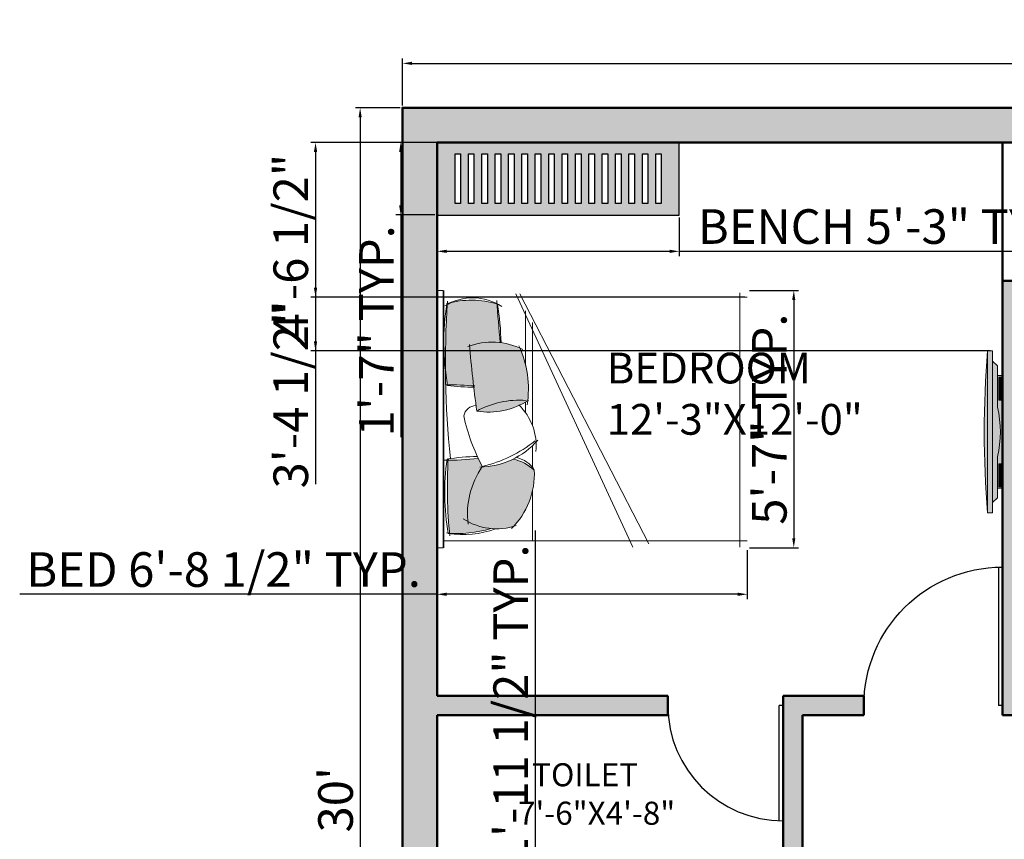
# Model space of a CAD drawing. Units: inches. Extents: x 3274 to 5176, y 1085 to 2172.
# Tile 6 of 16: x 3274 to 3530, y 1844 to 2057. Entities that reach past the tile are written whole.
import ezdxf

# ---------------------------------------------------------------- set-up
doc = ezdxf.new("R2010")
doc.units = ezdxf.units.IN
for name, color, linetype, lineweight in [('0.10', 252, 'Continuous', 9), ('A-ANNO-DIMS', 2, 'Continuous', 18), ('A-AREA-IDEN', 3, 'Continuous', 25), ('A-DOOR', 4, 'Continuous', 25), ('A-EQPM', 8, 'Continuous', 18), ('A-FLOR-PATT', 252, 'Continuous', 13), ('A-FURN', 8, 'Continuous', 18), ('A-WALL', 7, 'Continuous', 50), ('A-WALL-PATT', 8, 'Continuous', 13), ('moveis', 254, 'Continuous', 5), ('parede', 7, 'Continuous', 30)]:
    doc.layers.add(name, color=color, linetype=linetype, lineweight=lineweight)
doc.layers.add('MESA', color=7, linetype='Continuous')
doc.styles.get("Standard").update_dxf_attribs({"font": 'arial.ttf'})
doc.dimstyles.new('ISO-25', dxfattribs={"dimtxt": 9, "dimasz": 2.5, "dimexe": 1.25, "dimexo": 0.625, "dimtad": 1, "dimdec": 1, "dimlunit": 3, "dimtxsty": 'Standard', "dimcen": 2.5, "dimclrd": 4, "dimclre": 4, "dimclrt": 1, "dimadec": 0, "dimazin": 0, "dimtfac": 1, "dimtdec": 1, "dimtmove": 0, "dimatfit": 3, "dimfxl": 1, "dimarcsym": 0})

# ---------------------------------------------------------------- blocks, each defined once
blk = doc.blocks.new('1')
for p, q in [((0, 36), (0, 0)), ((1, 36), (1, 0)), ((0, 0), (1, 0))]:
    blk.add_line(p, q)
blk.add_arc((0, 0), 36, 0, 90)
blk = doc.blocks.new('2')
for p, q in [((0, 30), (0, 0)), ((1, 30), (1, 0)), ((0, 0), (1, 0))]:
    blk.add_line(p, q)
blk.add_arc((0, 0), 30, 0, 90)
blk = doc.blocks.new('*D67')
at = {"layer": 'A-ANNO-DIMS', "color": 0, "lineweight": -2, "transparency": 16777216}
for p, q in [((3373.3, 2035.11), (3373.3, 2047.29)), ((3375.8, 2046.04), (3730.8, 2046.04)), ((3733.3, 2035.11), (3733.3, 2047.29))]:
    blk.add_line(p, q, dxfattribs=at)
at = {"layer": 'A-ANNO-DIMS', "color": 0, "transparency": 16777216}
for points in [[(3375.8, 2046.46), (3375.8, 2045.63), (3373.3, 2046.04)], [(3730.8, 2046.46), (3730.8, 2045.63), (3733.3, 2046.04)]]:
    blk.add_solid(points, dxfattribs=at)
at = {"layer": 'Defpoints', "color": 0, "transparency": 16777216}
for p in [(3733.3, 2046.04), (3373.3, 2034.48), (3733.3, 2034.48)]:
    blk.add_point(p, dxfattribs=at)
at = {"layer": 'A-ANNO-DIMS', "color": 0, "transparency": 16777216, "insert": (3553.3, 2051.27), "char_height": 9, "attachment_point": 5}
blk.add_mtext("30'", dxfattribs=at)
blk = doc.blocks.new('*D68')
at = {"layer": 'A-ANNO-DIMS', "color": 0, "lineweight": -2, "transparency": 16777216}
for p, q in [((3372.68, 2034.48), (3361.05, 2034.48)), ((3362.3, 2031.98), (3362.3, 1676.98)), ((3372.68, 1674.48), (3361.05, 1674.48))]:
    blk.add_line(p, q, dxfattribs=at)
at = {"layer": 'A-ANNO-DIMS', "color": 0, "transparency": 16777216}
for points in [[(3361.88, 2031.98), (3362.71, 2031.98), (3362.3, 2034.48)], [(3361.88, 1676.98), (3362.71, 1676.98), (3362.3, 1674.48)]]:
    blk.add_solid(points, dxfattribs=at)
at = {"layer": 'Defpoints', "color": 0, "transparency": 16777216}
for p in [(3373.3, 2034.48), (3362.3, 1674.48), (3373.3, 1674.48)]:
    blk.add_point(p, dxfattribs=at)
at = {"layer": 'A-ANNO-DIMS', "color": 0, "transparency": 16777216, "insert": (3357.07, 1854.48), "char_height": 9, "attachment_point": 5, "rotation": 90}
blk.add_mtext("30'", dxfattribs=at)
blk = doc.blocks.new('camita')
at = {"layer": '0.10'}
for p, q in [((-0.85, -0.045), (0.85, -0.045)), ((-0.805, -0.045), (-0.805, -2.0485)), ((0.805, -0.045), (0.805, -2.0485)), ((-0.8271, -0.521), (0.8464, -1.2932)), ((-0.8271, -0.5476), (0.8236, -1.3992)), ((-0.7161, -0.585), (-0.3554, -0.585)), ((-0.1136, -0.585), (-0.0485, -0.585)), ((-0.638, -0.63), (0.0434, -0.63)), ((0.1749, -0.63), (0.3179, -0.63)), ((0.4739, -0.63), (0.805, -0.63)), ((-0.8354, -2), (0.8464, -2))]:
    blk.add_line(p, q, dxfattribs=at)
blk.add_lwpolyline([(-0.85, -0.0405), (0.85, -0.0405), (0.85, 0), (-0.85, 0)], close=True, dxfattribs=at)
for centre, radius, start, end in [((-0.4574, -0.2364), 0.3443, 147.50996, 213.83359), ((-0.1997, -0.2266), 0.5864, 163.92635, 197.14087), ((-0.3639, -5.8457), 5.7909, 83.80731, 94.12107), ((-0.5104, -1.7232), 1.6781, 80.12554, 98.66187), ((2.3534, -0.0532), 2.5803, 180.10628, 184.38541), ((-1.4396, -0.0609), 1.7117, 352.92911, 0.39592), ((0.4863, -1.6286), 1.5781, 80.16015, 98.05996), ((0.0294, -0.1377), 0.7262, 342.58415, 6.00484), ((-1.5443, -0.2452), 1.3333, 359.93941, 7.55329), ((1.5815, -0.2893), 1.3353, 170.38021, 178.99138), ((0.4524, -3.0675), 2.9996, 83.90257, 93.67595), ((0.1326, -0.1696), 0.6307, 339.92303, 8.74334), ((-0.007, -0.258), 0.0828, 100.01798, 179.73597), ((-0.2931, -1.4378), 1.2903, 61.97485, 77.84351), ((0.3203, -0.3944), 0.4043, 341.45245, 33.45121), ((-0.0543, -0.3633), 0.4542, 159.30257, 206.50263), ((-1.3301, -9.6748), 9.4985, 82.27078, 84.93989), ((0.6265, -0.7518), 0.5508, 82.96906, 124.67388), ((0.4585, -0.5454), 0.5842, 151.04555, 184.14969), ((-0.5341, -0.3393), 0.4875, 327.26442, 9.0473), ((-0.1986, -0.2742), 0.5159, 310.73945, 359.05759), ((-0.5673, -0.0868), 0.9057, 321.69527, 346.46261), ((-1.8672, -14.986), 14.6323, 84.65974, 85.75157), ((-0.4598, 1.4861), 1.9092, 260.95299, 268.65169), ((0.5707, -0.4317), 0.3145, 192.93877, 221.96363), ((0.3612, -0.133), 0.5096, 267.25889, 315.29965), ((-0.2002, 0.064), 0.6673, 244.78094, 279.06058), ((0.179, -0.272), 0.3828, 224.52836, 275.22287), ((0.4384, -0.4834), 0.1898, 193.68485, 236.70352)]:
    blk.add_arc(centre, radius, start, end, dxfattribs=at)
blk = doc.blocks.new('Banco Lintz')
at = {"layer": 'MESA', "ltscale": 0.05}
h = blk.add_hatch(color=256, dxfattribs=at)
h.dxf.hatch_style = 1
h.set_gradient(color1=(138, 84, 66), color2=(0, 0, 0), one_color=1, name='INVCYLINDER')
h.paths.add_polyline_path([(0.48, 0), (0, 0), (0, -1.6), (0.48, -1.6)])
h.paths.add_polyline_path([(0.4034, -0.5091), (0.0766, -0.5091), (0.0766, -0.4724), (0.4034, -0.4724)], flags=16)
h.paths.add_polyline_path([(0.4034, -0.5608), (0.4034, -0.5974), (0.0766, -0.5974), (0.0766, -0.5608)], flags=16)
h.paths.add_polyline_path([(0.4034, -0.4207), (0.0766, -0.4207), (0.0766, -0.384), (0.4034, -0.384)], flags=16)
h.paths.add_polyline_path([(0.4034, -0.6491), (0.4034, -0.6858), (0.0766, -0.6858), (0.0766, -0.6491)], flags=16)
h.paths.add_polyline_path([(0.4034, -0.3323), (0.0766, -0.3323), (0.0766, -0.2957), (0.4034, -0.2957)], flags=16)
h.paths.add_polyline_path([(0.4034, -0.7375), (0.4034, -0.7741), (0.0766, -0.7741), (0.0766, -0.7375)], flags=16)
h.paths.add_polyline_path([(0.4034, -0.244), (0.0766, -0.244), (0.0766, -0.2073), (0.4034, -0.2073)], flags=16)
h.paths.add_polyline_path([(0.4034, -0.8259), (0.4034, -0.8625), (0.0766, -0.8625), (0.0766, -0.8259)], flags=16)
h.paths.add_polyline_path([(0.4034, -0.1556), (0.0766, -0.1556), (0.0766, -0.119), (0.4034, -0.119)], flags=16)
h.paths.add_polyline_path([(0.4034, -0.9142), (0.4034, -0.9509), (0.0766, -0.9509), (0.0766, -0.9142)], flags=16)
h.paths.add_polyline_path([(0.4034, -1.0026), (0.4034, -1.0392), (0.0766, -1.0392), (0.0766, -1.0026)], flags=16)
h.paths.add_polyline_path([(0.4034, -1.0909), (0.4034, -1.1276), (0.0766, -1.1276), (0.0766, -1.0909)], flags=16)
h.paths.add_polyline_path([(0.4034, -1.1793), (0.4034, -1.216), (0.0766, -1.216), (0.0766, -1.1793)], flags=16)
h.paths.add_polyline_path([(0.4034, -1.2677), (0.4034, -1.3043), (0.0766, -1.3043), (0.0766, -1.2677)], flags=16)
h.paths.add_polyline_path([(0.4034, -1.356), (0.4034, -1.3927), (0.0766, -1.3927), (0.0766, -1.356)], flags=16)
h.paths.add_polyline_path([(0.4034, -1.4444), (0.4034, -1.481), (0.0766, -1.481), (0.0766, -1.4444)], flags=16)
for points in [[(0, -1.6), (0.48, -1.6), (0.48, 0), (0, 0)], [(0.0766, -0.119), (0.4034, -0.119), (0.4034, -0.1556), (0.0766, -0.1556)], [(0.0766, -0.2073), (0.4034, -0.2073), (0.4034, -0.244), (0.0766, -0.244)], [(0.0766, -0.2957), (0.4034, -0.2957), (0.4034, -0.3323), (0.0766, -0.3323)], [(0.0766, -0.384), (0.4034, -0.384), (0.4034, -0.4207), (0.0766, -0.4207)], [(0.0766, -0.4724), (0.4034, -0.4724), (0.4034, -0.5091), (0.0766, -0.5091)], [(0.0766, -0.5608), (0.4034, -0.5608), (0.4034, -0.5974), (0.0766, -0.5974)], [(0.0766, -0.6491), (0.4034, -0.6491), (0.4034, -0.6858), (0.0766, -0.6858)], [(0.0766, -0.7375), (0.4034, -0.7375), (0.4034, -0.7741), (0.0766, -0.7741)], [(0.0766, -0.8259), (0.4034, -0.8259), (0.4034, -0.8625), (0.0766, -0.8625)], [(0.0766, -0.9142), (0.4034, -0.9142), (0.4034, -0.9509), (0.0766, -0.9509)], [(0.0766, -1.0026), (0.4034, -1.0026), (0.4034, -1.0392), (0.0766, -1.0392)], [(0.0766, -1.0909), (0.4034, -1.0909), (0.4034, -1.1276), (0.0766, -1.1276)], [(0.0766, -1.1793), (0.4034, -1.1793), (0.4034, -1.216), (0.0766, -1.216)], [(0.0766, -1.2677), (0.4034, -1.2677), (0.4034, -1.3043), (0.0766, -1.3043)], [(0.0766, -1.356), (0.4034, -1.356), (0.4034, -1.3927), (0.0766, -1.3927)], [(0.0766, -1.4444), (0.4034, -1.4444), (0.4034, -1.481), (0.0766, -1.481)]]:
    blk.add_lwpolyline(points, close=True, dxfattribs=at)
blk = doc.blocks.new('PLASMA 2')
at = {"layer": 'moveis', "ltscale": 0.08}
h = blk.add_hatch(dxfattribs=at)
h.set_pattern_fill('_USER,_O', color=256, scale=0.008, double=1, pattern_type=0)
h.set_pattern_definition([(360, (-4.134502, -6.848382), (0, 0.008), []), (90, (-4.134502, -6.848382), (-0.008, 0), [])])
h.paths.add_polyline_path([(-0.2099, -0.0965), (-0.3623, -0.0965), (-0.3623, -0.1111), (-0.2099, -0.1111)])
h = blk.add_hatch(dxfattribs=at)
h.set_pattern_fill('_USER,_O', color=256, scale=0.008, double=1, pattern_type=0)
h.set_pattern_definition([(180, (4.134502, -6.848382), (0, 0.008), []), (90, (4.134502, -6.848382), (0.008, 0), [])])
h.paths.add_polyline_path([(0.2099, -0.0965), (0.3623, -0.0965), (0.3623, -0.1111), (0.2099, -0.1111)])
at = {"layer": 'parede', "ltscale": 0.08}
h = blk.add_hatch(color=256, dxfattribs=at)
h.dxf.hatch_style = 1
h.set_gradient(color1=(131, 136, 145), one_color=1, tint=1, name='CURVED')
h.paths.add_polyline_path([(-0.535, -0.0215), (0.535, -0.0215, 0.040195)])
h = blk.add_hatch(color=256, dxfattribs=at)
h.dxf.hatch_style = 1
h.set_gradient(color1=(131, 136, 145), color2=(0, 0, 0), one_color=1, name='CURVED')
h.paths.add_polyline_path([(0.535, -0.0215), (-0.535, -0.0215), (-0.535, -0.0553), (0.535, -0.0553)])
h = blk.add_hatch(color=256, dxfattribs=at)
h.dxf.hatch_style = 1
h.set_gradient(color1=(131, 136, 145), one_color=1, tint=1, name='CYLINDER')
h.paths.add_polyline_path([(0.4673, -0.0553), (-0.4673, -0.0553), (-0.4363, -0.0876), (-0.1636, -0.0876, 0.114423), (0.1636, -0.0876), (0.4363, -0.0876)])
h = blk.add_hatch(color=256, dxfattribs=at)
h.dxf.hatch_style = 1
h.set_gradient(color1=(131, 136, 145), color2=(0, 0, 0), one_color=1, name='CURVED')
h.paths.add_polyline_path([(0.3724, -0.0876), (0.1636, -0.0876, -0.114423), (-0.1636, -0.0876), (-0.3724, -0.0876), (-0.3724, -0.12), (0.3724, -0.12)])
h.paths.add_polyline_path([(-0.2099, -0.1111), (-0.3623, -0.1111), (-0.3623, -0.0965), (-0.2099, -0.0965)], flags=16)
h.paths.add_polyline_path([(0.2099, -0.1111), (0.2099, -0.0965), (0.3623, -0.0965), (0.3623, -0.1111)], flags=16)
at = {"layer": 'moveis', "ltscale": 0.08}
for p, q in [((-0.535, -0.0215), (-0.535, -0.0553)), ((-0.535, -0.0215), (0.535, -0.0215)), ((0.535, -0.0553), (-0.535, -0.0553)), ((-0.4673, -0.0553), (-0.4363, -0.0876)), ((0.4673, -0.0553), (0.4363, -0.0876)), ((0.535, -0.0553), (0.535, -0.0215)), ((-0.4363, -0.0876), (-0.1636, -0.0876)), ((-0.3724, -0.0876), (-0.3724, -0.12)), ((-0.3724, -0.12), (0.3724, -0.12)), ((0.1636, -0.0876), (0.4363, -0.0876)), ((0.3724, -0.0876), (0.3724, -0.12))]:
    blk.add_line(p, q, dxfattribs=at)
for points in [[(-0.3623, -0.0965), (-0.2099, -0.0965), (-0.2099, -0.1111), (-0.3623, -0.1111)], [(0.3623, -0.0965), (0.2099, -0.0965), (0.2099, -0.1111), (0.3623, -0.1111)]]:
    blk.add_lwpolyline(points, close=True, dxfattribs=at)
for centre, radius, start, end in [((0, -6.6658), 6.6658, 85.39647, 94.60353), ((0, 0.6178), 0.7242, 256.94486, 283.05514)]:
    blk.add_arc(centre, radius, start, end, dxfattribs=at)
blk = doc.blocks.new('*D132')
at = {"layer": 'A-ANNO-DIMS', "color": 4, "lineweight": -2, "transparency": 16777216}
for p, q in [((3382.3, 1919.39), (3382.3, 1906.67)), ((3462.96, 1919.39), (3462.96, 1906.67)), ((3382.3, 1907.92), (3273.77, 1907.92)), ((3460.46, 1907.92), (3384.8, 1907.92))]:
    blk.add_line(p, q, dxfattribs=at)
at = {"layer": 'A-ANNO-DIMS', "color": 4, "transparency": 16777216}
for points in [[(3384.8, 1908.33), (3384.8, 1907.5), (3382.3, 1907.92)], [(3460.46, 1908.33), (3460.46, 1907.5), (3462.96, 1907.92)]]:
    blk.add_solid(points, dxfattribs=at)
at = {"layer": 'Defpoints', "color": 0, "transparency": 16777216}
for p in [(3382.3, 1920.01), (3462.96, 1920.01), (3382.3, 1907.92)]:
    blk.add_point(p, dxfattribs=at)
at = {"layer": 'A-ANNO-DIMS', "color": 1, "transparency": 16777216, "insert": (3326.79, 1913.19), "char_height": 9, "attachment_point": 5}
blk.add_mtext('BED 6\'-8 1/2" TYP.', dxfattribs=at)
blk = doc.blocks.new('*D133')
at = {"layer": 'A-ANNO-DIMS', "color": 4, "lineweight": -2, "transparency": 16777216}
for p, q in [((3463.58, 1986.95), (3476.31, 1986.95)), ((3475.06, 1984.45), (3475.06, 1922.51)), ((3463.58, 1920.01), (3476.31, 1920.01))]:
    blk.add_line(p, q, dxfattribs=at)
at = {"layer": 'A-ANNO-DIMS', "color": 4, "transparency": 16777216}
for points in [[(3474.64, 1984.45), (3475.47, 1984.45), (3475.06, 1986.95)], [(3474.64, 1922.51), (3475.47, 1922.51), (3475.06, 1920.01)]]:
    blk.add_solid(points, dxfattribs=at)
at = {"layer": 'Defpoints', "color": 0, "transparency": 16777216}
for p in [(3462.96, 1986.95), (3462.96, 1920.01), (3475.06, 1920.01)]:
    blk.add_point(p, dxfattribs=at)
at = {"layer": 'A-ANNO-DIMS', "color": 1, "transparency": 16777216, "insert": (3469.86, 1953.48), "char_height": 9, "attachment_point": 5, "rotation": 90}
blk.add_mtext('5\'-7" TYP.', dxfattribs=at)
blk = doc.blocks.new('*D144')
at = {"layer": 'A-ANNO-DIMS', "color": 4, "lineweight": -2, "transparency": 16777216}
for p, q in [((3382.3, 2005.96), (3382.3, 1995.89)), ((3445.29, 2005.96), (3445.29, 1995.89)), ((3384.8, 1997.14), (3442.79, 1997.14)), ((3445.29, 1997.14), (3551.01, 1997.14))]:
    blk.add_line(p, q, dxfattribs=at)
at = {"layer": 'A-ANNO-DIMS', "color": 4, "transparency": 16777216}
for points in [[(3384.8, 1997.55), (3384.8, 1996.72), (3382.3, 1997.14)], [(3442.79, 1997.55), (3442.79, 1996.72), (3445.29, 1997.14)]]:
    blk.add_solid(points, dxfattribs=at)
at = {"layer": 'Defpoints', "color": 0, "transparency": 16777216}
for p in [(3382.3, 2006.59), (3445.29, 2006.59), (3445.29, 1997.14)]:
    blk.add_point(p, dxfattribs=at)
at = {"layer": 'A-ANNO-DIMS', "color": 1, "transparency": 16777216, "insert": (3499.4, 2002.42), "char_height": 9, "attachment_point": 5}
blk.add_mtext('BENCH 5\'-3" TYP.', dxfattribs=at)
blk = doc.blocks.new('*D145')
at = {"layer": 'A-ANNO-DIMS', "color": 4, "lineweight": -2, "transparency": 16777216}
for p, q in [((3381.68, 2025.48), (3371.6, 2025.48)), ((3372.85, 2022.98), (3372.85, 2009.09)), ((3381.68, 2006.59), (3371.6, 2006.59)), ((3372.85, 2006.59), (3372.85, 1948.82))]:
    blk.add_line(p, q, dxfattribs=at)
at = {"layer": 'A-ANNO-DIMS', "color": 4, "transparency": 16777216}
for points in [[(3372.44, 2022.98), (3373.27, 2022.98), (3372.85, 2025.48)], [(3372.44, 2009.09), (3373.27, 2009.09), (3372.85, 2006.59)]]:
    blk.add_solid(points, dxfattribs=at)
at = {"layer": 'Defpoints', "color": 0, "transparency": 16777216}
for p in [(3382.3, 2025.48), (3372.85, 2006.59), (3382.3, 2006.59)]:
    blk.add_point(p, dxfattribs=at)
at = {"layer": 'A-ANNO-DIMS', "color": 1, "transparency": 16777216, "insert": (3367.71, 1976.45), "char_height": 9, "attachment_point": 5, "rotation": 90}
blk.add_mtext('1\'-7" TYP.', dxfattribs=at)
blk = doc.blocks.new('*D146')
at = {"layer": 'A-ANNO-DIMS', "color": 4, "lineweight": -2, "transparency": 16777216}
for p, q in [((3407.89, 1746.82), (3407.89, 1924.51)), ((3404.98, 1746.82), (3409.14, 1746.82)), ((3407.89, 1725.73), (3407.89, 1744.32)), ((3404.98, 1723.23), (3409.14, 1723.23))]:
    blk.add_line(p, q, dxfattribs=at)
at = {"layer": 'A-ANNO-DIMS', "color": 4, "transparency": 16777216}
for points in [[(3407.48, 1744.32), (3408.31, 1744.32), (3407.89, 1746.82)], [(3407.48, 1725.73), (3408.31, 1725.73), (3407.89, 1723.23)]]:
    blk.add_solid(points, dxfattribs=at)
at = {"layer": 'Defpoints', "color": 0, "transparency": 16777216}
for p in [(3404.36, 1746.82), (3407.89, 1746.82), (3404.36, 1723.23)]:
    blk.add_point(p, dxfattribs=at)
at = {"layer": 'A-ANNO-DIMS', "color": 1, "transparency": 16777216, "insert": (3402.62, 1836.92), "char_height": 9, "attachment_point": 5, "rotation": 90}
blk.add_mtext('KITCHEN SINK 1\'-11 1/2" TYP.', dxfattribs=at)
blk = doc.blocks.new('*D176')
at = {"layer": 'A-ANNO-DIMS', "color": 4, "lineweight": -2, "transparency": 16777216}
for p, q in [((3381.68, 2025.48), (3349.45, 2025.48)), ((3350.7, 2022.98), (3350.7, 1987.68)), ((3462.33, 1985.18), (3349.45, 1985.18)), ((3350.7, 1985.18), (3350.7, 1936.54))]:
    blk.add_line(p, q, dxfattribs=at)
at = {"layer": 'A-ANNO-DIMS', "color": 4, "transparency": 16777216}
for points in [[(3350.28, 2022.98), (3351.12, 2022.98), (3350.7, 2025.48)], [(3350.28, 1987.68), (3351.12, 1987.68), (3350.7, 1985.18)]]:
    blk.add_solid(points, dxfattribs=at)
at = {"layer": 'Defpoints', "color": 0, "transparency": 16777216}
for p in [(3382.3, 2025.48), (3350.7, 1985.18), (3462.96, 1985.18)]:
    blk.add_point(p, dxfattribs=at)
at = {"layer": 'A-ANNO-DIMS', "color": 1, "transparency": 16777216, "insert": (3345.42, 1959.61), "char_height": 9, "attachment_point": 5, "rotation": 90}
blk.add_mtext('3\'-4 1/2"', dxfattribs=at)
blk = doc.blocks.new('*D178')
at = {"layer": 'A-ANNO-DIMS', "color": 4, "lineweight": -2, "transparency": 16777216}
for p, q in [((3528.68, 2025.48), (3349.45, 2025.48)), ((3350.7, 2022.98), (3350.7, 1973.71)), ((3526.13, 1971.21), (3349.45, 1971.21))]:
    blk.add_line(p, q, dxfattribs=at)
at = {"layer": 'A-ANNO-DIMS', "color": 4, "transparency": 16777216}
for points in [[(3350.28, 2022.98), (3351.12, 2022.98), (3350.7, 2025.48)], [(3350.28, 1973.71), (3351.12, 1973.71), (3350.7, 1971.21)]]:
    blk.add_solid(points, dxfattribs=at)
at = {"layer": 'Defpoints', "color": 0, "transparency": 16777216}
for p in [(3529.3, 2025.48), (3350.7, 1971.21), (3526.75, 1971.21)]:
    blk.add_point(p, dxfattribs=at)
at = {"layer": 'A-ANNO-DIMS', "color": 1, "transparency": 16777216, "insert": (3345.42, 1998.35), "char_height": 9, "attachment_point": 5, "rotation": 90}
blk.add_mtext('4\'-6 1/2"', dxfattribs=at)

msp = doc.modelspace()

# ---------------------------------------------------------------- hatches: boundary and pattern name
at = {"layer": 'A-FLOR-PATT'}
h = msp.add_hatch(color=256, dxfattribs=at)
h.dxf.hatch_style = 1
h.paths.add_polyline_path([(3397.88, 1983.45, 0.131047), (3385.98, 1983.83, 0.020657), (3384.99, 1983.33, 0.01851), (3384.46, 1966.46, 0.015442), (3385.03, 1962.42, -0.016701), (3391.81, 1962.15, -0.006967), (3390.73, 1972.51, -0.113891), (3398.73, 1973.38, -0.004387)])
h.paths.add_polyline_path([(3394.07, 1941.15, -0.011742), (3393, 1943.28, -0.029051), (3385.19, 1942.77, 0.040212), (3385.57, 1923.81, 0.094792), (3396.25, 1925.03, -0.098488), (3390.31, 1926.84, -0.175864)])
h.paths.add_polyline_path([(3403.81, 1971.99, 0.189536), (3390.73, 1972.51, 0.011408), (3392.64, 1955.56, 0.181694), (3405.87, 1958.26, 0.134508)])
h.paths.add_polyline_path([(3407.58, 1940.22, 0.127326), (3402.07, 1943.08, -0.104045), (3393.97, 1941.01, 0.173835), (3390.31, 1926.84, 0.194952), (3402.2, 1925.56, 0.202559)])
at = {"layer": 'A-WALL-PATT'}
h = msp.add_hatch(color=256, dxfattribs=at)
h.dxf.hatch_style = 1
h.paths.add_polyline_path([(3733.3, 2034.48), (3373.3, 2034.48), (3373.3, 1674.48), (3406.3, 1674.48), (3406.3, 1683.48), (3382.3, 1683.48), (3382.3, 1767.48), (3442.3, 1767.48), (3442.3, 1772.48), (3382.3, 1772.48), (3382.3, 1876.48), (3442.3, 1876.48), (3442.3, 1881.48), (3382.3, 1881.48), (3382.3, 2025.48), (3724.3, 2025.48), (3724.3, 1881.48), (3594.3, 1881.48), (3594.3, 1876.48), (3724.3, 1876.48), (3724.3, 1776.48), (3656.3, 1776.48), (3656.3, 1767.48), (3724.3, 1767.48), (3724.3, 1683.48), (3682.3, 1683.48), (3682.3, 1674.48), (3733.3, 1674.48)])
h.paths.add_polyline_path([(3477.3, 1876.48), (3493.3, 1876.48), (3493.3, 1881.48), (3472.3, 1881.48), (3472.3, 1820.48), (3417.3, 1820.48), (3417.3, 1840.48), (3412.3, 1840.48), (3412.3, 1815.48), (3472.3, 1815.48), (3472.3, 1767.48), (3493.3, 1767.48), (3493.3, 1772.48), (3477.3, 1772.48)], flags=17)
h.paths.add_polyline_path([(3534.3, 1984.48), (3552.3, 1984.48), (3552.3, 1989.48), (3529.3, 1989.48), (3529.3, 1876.48), (3552.3, 1876.48), (3552.3, 1881.48), (3534.3, 1881.48), (3534.3, 1919.48), (3564.3, 1919.48), (3564.3, 1924.48), (3534.3, 1924.48)], flags=17)
h.paths.add_polyline_path([(3599.3, 1989.48), (3576.3, 1989.48), (3576.3, 1984.48), (3594.3, 1984.48), (3594.3, 1917.48), (3599.3, 1917.48)], flags=17)
h.paths.add_polyline_path([(3534.3, 1767.48), (3539.3, 1767.48), (3539.3, 1776.48), (3529.3, 1776.48), (3529.3, 1683.48), (3478.3, 1683.48), (3478.3, 1674.48), (3534.3, 1674.48)], flags=17)
h.paths.add_polyline_path([(3596.3, 1776.48), (3587.3, 1776.48), (3587.3, 1771.98), (3587.3, 1767.48), (3596.3, 1767.48)], flags=17)
h.paths.add_polyline_path([(3610.3, 1683.48), (3594.3, 1683.48), (3594.3, 1674.48), (3610.3, 1674.48)], flags=17)
h.paths.add_polyline_path([(3589.35, 1817.42), (3663.55, 1817.42), (3663.55, 1847.27), (3589.35, 1847.27)], flags=25)
h.paths.add_polyline_path([(3545.54, 1954.13), (3584.72, 1954.13), (3584.72, 1976.52), (3545.54, 1976.52)], flags=25)
h.paths.add_polyline_path([(3635.11, 1944.89), (3703.51, 1944.89), (3703.51, 1974.74), (3635.11, 1974.74)], flags=25)
h.paths.add_polyline_path([(3543.78, 1998.17), (3585.75, 1998.17), (3585.75, 2020.56), (3543.78, 2020.56)], flags=25)
h.paths.add_polyline_path([(3423.19, 1944.89), (3491.58, 1944.89), (3491.58, 1974.74), (3423.19, 1974.74)], flags=25)

# ---------------------------------------------------------------- linework, layer by layer
at = {"layer": 'A-WALL'}
for p, q in [((3382.3, 2025.48), (3724.3, 2025.48)), ((3382.3, 1881.48), (3382.3, 2025.48)), ((3529.3, 1876.48), (3529.3, 2025.48)), ((3529.3, 1989.48), (3599.3, 1989.48)), ((3382.3, 1881.48), (3442.3, 1881.48)), ((3442.3, 1876.48), (3442.3, 1881.48)), ((3472.3, 1881.48), (3493.3, 1881.48)), ((3472.3, 1820.48), (3472.3, 1881.48)), ((3493.3, 1876.48), (3493.3, 1881.48)), ((3382.3, 1876.48), (3442.3, 1876.48)), ((3382.3, 1772.48), (3382.3, 1876.48)), ((3477.3, 1876.48), (3493.3, 1876.48)), ((3477.3, 1772.48), (3477.3, 1876.48)), ((3529.3, 1876.48), (3552.3, 1876.48))]:
    msp.add_line(p, q, dxfattribs=at)
msp.add_lwpolyline([(3534.3, 1674.48), (3373.3, 1674.48), (3373.3, 2034.48), (3733.3, 2034.48), (3733.3, 1674.48), (3594.3, 1674.48)], dxfattribs=at)

# ---------------------------------------------------------------- block references
at = {"layer": 'A-DOOR', "xscale": -1}
msp.add_blockref('1', (3529.3, 1878.98), dxfattribs=at)
at = {"layer": 'A-DOOR', "rotation": 180}
msp.add_blockref('2', (3472.3, 1878.98), dxfattribs=at)
at = {"layer": 'A-EQPM', "xscale": 39.37, "yscale": 39.37, "zscale": 39.37, "rotation": 90}
msp.add_blockref('PLASMA 2', (3524.58, 1950.15), dxfattribs=at)
at = {"layer": 'A-FURN'}
for name, p, xscale, yscale, zscale, rotation in [('Banco Lintz', (3445.29, 2025.48), 39.37, 39.37, 39.37, 270), ('camita', (3382.3, 1953.48), -39.375, 39.375, 39.375, 90)]:
    msp.add_blockref(name, p, dxfattribs=dict(at, xscale=xscale, yscale=yscale, zscale=zscale, rotation=rotation))

# ---------------------------------------------------------------- texts
at = {"layer": 'A-AREA-IDEN', "attachment_point": 1}
for s, heights, insert, char_height in [('BEDROOM\\P12\'-3"X12\'-0"', [0], (3426.41, 1970.76), 8), ('  TOILET\\P7\'-6"X4\'-8"', [16.24], (3403.37, 1863.96), 6)]:
    msp.add_mtext_dynamic_manual_height_columns(s, width=58.0121, gutter_width=30, heights=heights, dxfattribs=dict(at, insert=insert, char_height=char_height))

# ---------------------------------------------------------------- dimensions: what is measured, and where the dimension line sits
at = {"layer": 'A-ANNO-DIMS'}
dim = msp.add_linear_dim(base=(3733.3, 2046.04), p1=(3373.3, 2034.48), p2=(3733.3, 2034.48), dimstyle='ISO-25', override={"dimclrd": 0, "dimclre": 0, "dimclrt": 0}, dxfattribs=at)
dim.commit()
dim.dimension.update_dxf_attribs({"geometry": '*D67', "text_midpoint": (3553.3, 2051.27)})
for base, p1, p2, override, picture, middle in [((3362.3, 1674.48), (3373.3, 2034.48), (3373.3, 1674.48), {"dimclrd": 0, "dimclre": 0, "dimclrt": 0}, '*D68', (3357.07, 1854.48)), ((3350.7, 1985.18), (3382.3, 2025.48), (3462.96, 1985.18), {"dimdec": 1, "dimlfac": 1, "dimrnd": 0, "dimzin": 1, "dimdsep": 46, "dimlunit": 4, "dimfrac": 2}, '*D176', (3345.42, 1959.61)), ((3350.7, 1971.21), (3529.3, 2025.48), (3526.75, 1971.21), {"dimdec": 1, "dimlfac": 1, "dimrnd": 0, "dimzin": 1, "dimdsep": 46, "dimlunit": 4, "dimfrac": 2}, '*D178', (3345.42, 1998.35))]:
    dim = msp.add_linear_dim(base=base, p1=p1, p2=p2, angle=90, dimstyle='ISO-25', override=override, dxfattribs=at)
    dim.commit()
    dim.dimension.update_dxf_attribs({"geometry": picture, "text_midpoint": middle})
for base, p1, p2, angle, text, picture, middle in [((3372.85, 2006.59), (3382.3, 2025.48), (3382.3, 2006.59), 270, '<> TYP.', '*D145', (3367.71, 1976.45)), ((3475.06, 1920.01), (3462.96, 1986.95), (3462.96, 1920.01), 270, '<> TYP.', '*D133', (3469.86, 1953.48)), ((3382.3, 1907.92), (3462.96, 1920.01), (3382.3, 1920.01), 180, 'BED <> TYP.', '*D132', (3326.79, 1913.19)), ((3407.89, 1746.82), (3404.36, 1723.23), (3404.36, 1746.82), 90, 'KITCHEN SINK <> TYP.', '*D146', (3402.62, 1836.92))]:
    dim = msp.add_linear_dim(base=base, p1=p1, p2=p2, angle=angle, text=text, dimstyle='ISO-25', override={"dimdec": 1, "dimrnd": 0, "dimzin": 1, "dimlunit": 4, "dimfrac": 2}, dxfattribs=at)
    dim.commit()
    dim.dimension.update_dxf_attribs({"geometry": picture, "text_midpoint": middle})
dim = msp.add_linear_dim(base=(3445.29, 1997.14), p1=(3382.3, 2006.59), p2=(3445.29, 2006.59), text='BENCH <> TYP.', dimstyle='ISO-25', override={"dimdec": 1, "dimrnd": 0, "dimzin": 1, "dimlunit": 4, "dimfrac": 2}, dxfattribs=at)
dim.commit()
dim.dimension.update_dxf_attribs({"geometry": '*D144', "text_midpoint": (3499.4, 2002.42)})

doc.saveas('drawing.dxf')
